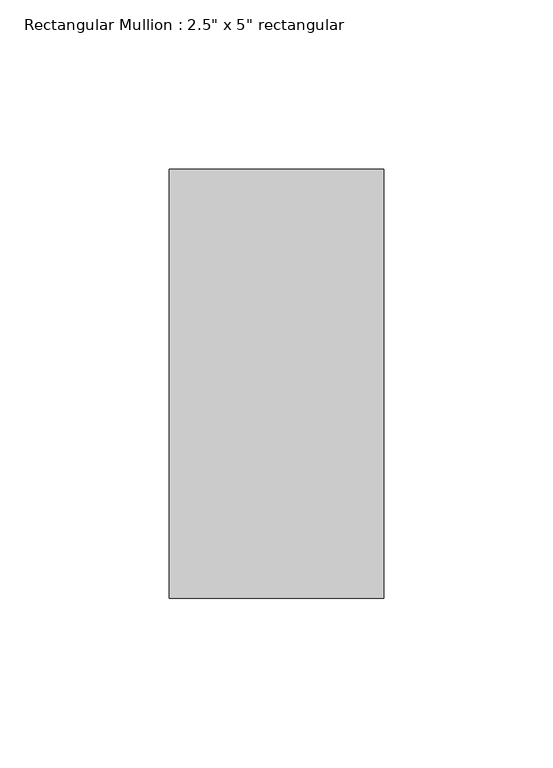
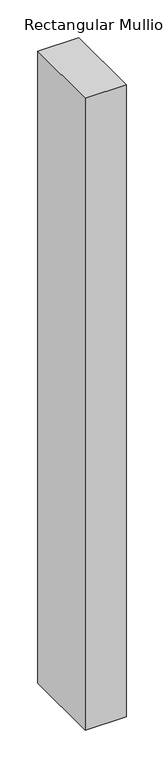
"""IFC4 building model written with IfcOpenShell, lengths in millimetres: member geometry."""

from ifc_helpers import new_model, si_unit, frame, origin, place, context, project, spatial, polyline, outline, extrude, source, transform, mapped, element, save


def member_bc9734be(model_context):
    return source(origin(), model_context, "Body", "SweptSolid", [
        extrude(outline(polyline([(31.75, 63.5), (31.75, -63.5), (-31.75, -63.5), (-31.75, 63.5), (31.75, 63.5)])), frame((0.0, 0.0, -1028.434107), z_axis=(0.0, 0.0, 1.0), x_axis=(1.0, 0.0, 0.0)), (0.0, 0.0, 1.0), 1028.434107),
    ])


if __name__ == "__main__":
    model = new_model("IFC4")
    model_context = context("Model", 3, world=origin())
    ifc_project = project(units=[si_unit("LENGTHUNIT", "METRE", prefix="MILLI")], contexts=[model_context])
    site = spatial("IfcSite", under=ifc_project)
    building = spatial("IfcBuilding", under=site)
    placement = place(None, origin())
    member_shape = member_bc9734be(model_context)
    element("IfcMember", 1, ObjectType="Rectangular Mullion : 2.5\" x 5\" rectangular", at=placement, inside=building, context=model_context, shape_type="MappedRepresentation", body=[
        mapped(member_shape, transform((0.0, 0.0, 0.0), x_axis=(1.0, 0.0, 0.0), y_axis=(0.0, 1.0, 0.0), z_axis=(0.0, 0.0, 1.0))),
    ])
    save(model, "model.ifc")

# Revit data of these elements
# Type "Rectangular Mullion : 2.5\" x 5\" rectangular"
#   built-in parameter 1007304 = 0.416667 (stored number, unit not read)
#   built-in parameter 1007301 = 0.104167 (stored number, unit not read)
#   built-in parameter 1007300 = 0.104167 (stored number, unit not read)
# Element 1 (IfcMember, "Rectangular Mullion : 2.5\" x 5\" rectangular")
#   Materials on its faces: "Roofing, EPDM Membrane"
# Materials
#   "Roofing, EPDM Membrane": class "Generic", colour RGB 127 127 127, transparency 0, Description = "EPDM roof membrane", Cost = 0
